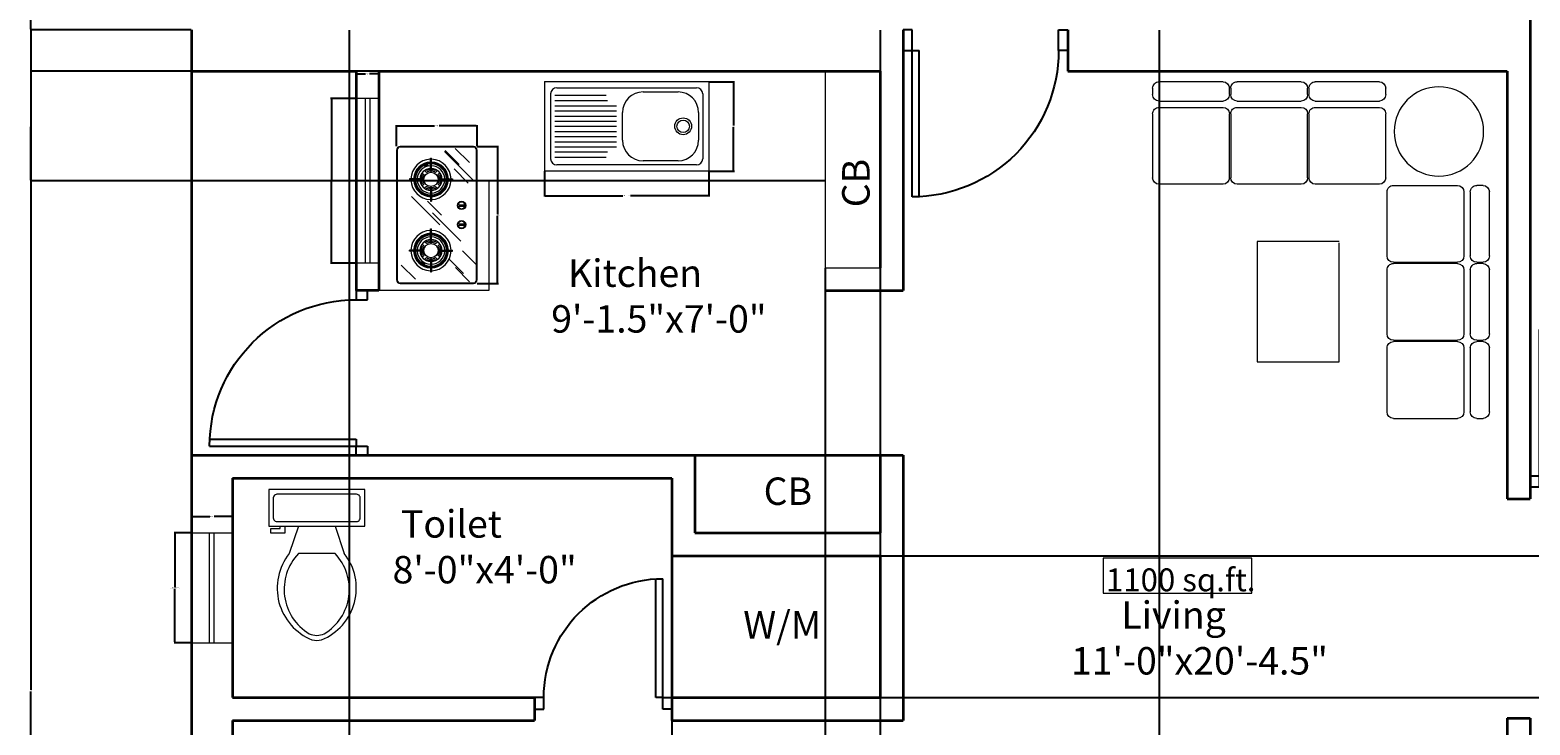
# Model space of a CAD drawing. Units: inches. Extents: x 3198 to 3702, y 1509 to 2253.
# Tile 2 of 6: x 3198 to 3526, y 1693 to 1845. Entities that reach past the tile are written whole.
import ezdxf

# ---------------------------------------------------------------- set-up
doc = ezdxf.new("R2010")
doc.units = ezdxf.units.IN
for name, color, linetype, lineweight in [('A-ANNO-DIMS', 2, 'Continuous', 18), ('A-ANNO-TEXT', 7, 'Continuous', 18), ('A-AREA-IDEN', 7, 'Continuous', 18), ('A-DOOR', 3, 'Continuous', 25), ('A-EQPM', 8, 'Continuous', 18), ('A-FLOR-CASE', 9, 'Continuous', 18), ('A-FLOR-FIXT', 9, 'Continuous', 18), ('A-FURN', 8, 'Continuous', 13), ('A-GLAZ', 4, 'Continuous', 18), ('A-WALL', 7, 'Continuous', 35)]:
    doc.layers.add(name, color=color, linetype=linetype, lineweight=lineweight)
doc.styles.get("Standard").update_dxf_attribs({"font": 'arial.ttf'})
doc.dimstyles.get("Standard").update_dxf_attribs({"dimtxt": 0.18, "dimasz": 0.18, "dimexe": 0.18, "dimexo": 0.0625, "dimgap": 0.09, "dimtad": 0, "dimtih": 1, "dimtoh": 1, "dimdec": 4, "dimzin": 0, "dimdsep": 46, "dimtxsty": 'Standard', "dimcen": 0.09, "dimadec": 0, "dimazin": 0, "dimtfac": 1, "dimtdec": 4, "dimtofl": 0, "dimtmove": 0, "dimatfit": 3, "dimfxl": 1, "dimtolj": 1, "dimtzin": 0, "dimarcsym": 0})

# ---------------------------------------------------------------- blocks, each defined once
blk = doc.blocks.new('A$C753D6792')
at = {"linetype": 'ByBlock'}
for p, q in [((0, 2530), (0, 2580)), ((50, 2630), (550, 2630)), ((600, 2580), (600, 2530)), ((610, 2530), (610, 2580)), ((660, 2630), (1160, 2630)), ((1210, 2580), (1210, 2530)), ((1220, 2530), (1220, 2580)), ((1270, 2630), (1770, 2630)), ((1820, 2580), (1820, 2530)), ((550, 2480), (50, 2480)), ((1160, 2480), (660, 2480)), ((1770, 2480), (1270, 2480)), ((0, 1880), (0, 2380)), ((550, 2430), (50, 2430)), ((600, 2380), (600, 1880)), ((610, 1880), (610, 2380)), ((1160, 2430), (660, 2430)), ((1210, 2380), (1210, 1880)), ((1220, 1880), (1220, 2380)), ((1770, 2430), (1270, 2430)), ((1820, 1880), (1820, 2380)), ((50, 1830), (427, 1830)), ((387, 1830), (550, 1830)), ((660, 1830), (1037, 1830)), ((997, 1830), (1160, 1830)), ((1270, 1830), (1647, 1830)), ((1607, 1830), (1770, 1830)), ((1830, 1770), (1830, 1393)), ((1880, 1820), (2380, 1820)), ((2430, 1270), (2430, 1770)), ((2480, 1270), (2480, 1770)), ((2530, 1820), (2580, 1820)), ((2630, 1770), (2630, 1270)), ((442, 815), (442, 1455)), ((442, 1455), (1372, 1455)), ((1382, 1455), (1382, 815)), ((1830, 1433), (1830, 1270)), ((2380, 1220), (1880, 1220)), ((1880, 1210), (2380, 1210)), ((2580, 1220), (2530, 1220)), ((2530, 1210), (2580, 1210)), ((1830, 1160), (1830, 783)), ((2430, 660), (2430, 1160)), ((2480, 660), (2480, 1160)), ((2630, 1160), (2630, 660)), ((1830, 823), (1830, 660)), ((1382, 815), (442, 815)), ((2380, 610), (1880, 610)), ((1880, 600), (2380, 600)), ((2580, 610), (2530, 610)), ((2530, 600), (2580, 600)), ((1830, 550), (1830, 173)), ((2430, 50), (2430, 550)), ((2480, 50), (2480, 550)), ((2630, 550), (2630, 50)), ((1830, 213), (1830, 50)), ((2380, 0), (1880, 0)), ((2580, 0), (2530, 0))]:
    blk.add_line(p, q, dxfattribs=at)
blk.add_circle((2242, 2235), 349, dxfattribs=at)
for centre, start, end in [((50, 2580), 90, 180), ((550, 2580), 0, 90), ((550, 2580), 0, 90), ((660, 2580), 90, 180), ((1160, 2580), 0, 90), ((1160, 2580), 0, 90), ((1270, 2580), 90, 180), ((1770, 2580), 0, 90), ((1770, 2580), 0, 90), ((50, 2530), 180, 270), ((550, 2530), 270, 0), ((550, 2530), 270, 0), ((660, 2530), 180, 270), ((1160, 2530), 270, 0), ((1160, 2530), 270, 0), ((1270, 2530), 180, 270), ((1770, 2530), 270, 0), ((1770, 2530), 270, 0), ((50, 2380), 90, 180), ((550, 2380), 0, 90), ((550, 2380), 0, 90), ((660, 2380), 90, 180), ((1160, 2380), 0, 90), ((1160, 2380), 0, 90), ((1270, 2380), 90, 180), ((1770, 2380), 0, 90), ((1770, 2380), 0, 90), ((50, 1880), 180, 270), ((550, 1880), 270, 0), ((660, 1880), 180, 270), ((1160, 1880), 270, 0), ((1270, 1880), 180, 270), ((1770, 1880), 270, 0), ((1880, 1770), 90, 180), ((2380, 1770), 0, 90), ((2530, 1770), 90, 180), ((2580, 1770), 0, 90), ((1880, 1270), 180, 270), ((1880, 1160), 90, 180), ((2380, 1270), 270, 0), ((2380, 1270), 270, 0), ((2380, 1160), 0, 90), ((2530, 1270), 180, 270), ((2530, 1270), 180, 270), ((2530, 1160), 90, 180), ((2580, 1270), 270, 0), ((2580, 1270), 270, 0), ((2580, 1160), 0, 90), ((1880, 660), 180, 270), ((1880, 550), 90, 180), ((2380, 660), 270, 0), ((2380, 660), 270, 0), ((2380, 550), 0, 90), ((2530, 660), 180, 270), ((2530, 660), 180, 270), ((2530, 550), 90, 180), ((2580, 660), 270, 0), ((2580, 660), 270, 0), ((2580, 550), 0, 90), ((1880, 50), 180, 270), ((2380, 50), 270, 0), ((2380, 50), 270, 0), ((2530, 50), 180, 270), ((2530, 50), 180, 270), ((2580, 50), 270, 0), ((2580, 50), 270, 0)]:
    blk.add_arc(centre, 50, start, end, dxfattribs=at)
blk = doc.blocks.new('A$C48FA29D1')
for p, q in [((23.9, 336.8), (101.3, 414.2)), ((177.6, 369.5), (182.6, 369.5)), ((320.9, 202.7), (475.7, 357.5)), ((572.4, 369.5), (567.4, 369.5)), ((63.2, 254.2), (63.2, 249.2)), ((299, 254.2), (299, 249.2)), ((374.2, 193.8), (451.6, 271.2)), ((451, 254.2), (451, 249.2)), ((686.8, 254.2), (686.8, 249.2)), ((232.1, 89.3), (386.9, 244.1)), ((567.6, 22.2), (722.4, 177)), ((650.5, 97.2), (727.9, 174.6)), ((10.1, 41), (87.5, 118.4)), ((54.5, 73.5), (131.9, 150.9)), ((177.6, 133.3), (182.6, 133.3)), ((549.9, 47.9), (627.2, 125.3)), ((572.4, 133.3), (567.4, 133.3)), ((661.4, 42), (738.7, 119.3)), ((100.9, 1.5), (178.3, 78.9))]:
    blk.add_line(p, q)
at = {"ltscale": 0.18}
for p, q in [((177.6, 296.7), (177.6, 369.5)), ((182.6, 296.7), (182.6, 369.5)), ((567.4, 296.7), (567.4, 369.5)), ((572.4, 296.7), (572.4, 369.5)), ((135.1, 254.2), (63.2, 254.2)), ((135.1, 249.2), (63.2, 249.2)), ((126.9, 279.5), (132.1, 274.3)), ((131.2, 286.5), (142, 275.7)), ((145.3, 300.6), (156.1, 289.8)), ((152.3, 304.9), (157.6, 299.7)), ((202.6, 299.7), (207.8, 304.9)), ((204, 289.8), (214.8, 300.6)), ((218.2, 275.7), (229, 286.5)), ((225, 254.2), (299, 254.2)), ((225, 249.2), (299, 249.2)), ((228.1, 274.3), (233.3, 279.5)), ((525, 254.2), (451, 254.2)), ((525, 249.2), (451, 249.2)), ((521.9, 274.3), (516.7, 279.5)), ((531.8, 275.7), (521, 286.5)), ((546, 289.8), (535.2, 300.6)), ((547.4, 299.7), (542.2, 304.9)), ((597.7, 304.9), (592.4, 299.7)), ((604.7, 300.6), (593.9, 289.8)), ((618.8, 286.5), (608, 275.7)), ((614.9, 254.2), (686.8, 254.2)), ((614.9, 249.2), (686.8, 249.2)), ((623.1, 279.5), (617.9, 274.3)), ((126.9, 224), (132.1, 229.2)), ((131.2, 217), (142, 227.8)), ((145.3, 202.8), (156.1, 213.6)), ((152.3, 198.5), (157.6, 203.8)), ((177.6, 206.8), (177.6, 133.3)), ((182.6, 206.8), (182.6, 133.3)), ((202.6, 203.8), (207.8, 198.5)), ((204, 213.6), (214.8, 202.8)), ((218.2, 227.8), (229, 217)), ((228.1, 229.2), (233.3, 224)), ((521.9, 229.2), (516.7, 224)), ((531.8, 227.8), (521, 217)), ((546, 213.6), (535.2, 202.8)), ((547.4, 203.8), (542.2, 198.5)), ((567.4, 206.8), (567.4, 133.3)), ((572.4, 206.8), (572.4, 133.3)), ((597.7, 198.5), (592.4, 203.8)), ((604.7, 202.8), (593.9, 213.6)), ((618.8, 217), (608, 227.8)), ((623.1, 224), (617.9, 229.2)), ((318.6, 99.8), (318.6, 69)), ((326.6, 99.8), (326.6, 69)), ((423.4, 99.8), (423.4, 69)), ((431.4, 99.8), (431.4, 69))]:
    blk.add_line(p, q, dxfattribs=at)
for points in [[(20, 0), (730, 0, 0.414214), (750, 20), (750, 420, 0.414214), (730, 440), (20, 440, 0.414214), (0, 420), (0, 20, 0.414214)], [(20, 3), (730, 3, 0.414214), (747, 20), (747, 420, 0.414214), (730, 437), (20, 437, 0.414214), (3, 420), (3, 20, 0.414214)]]:
    blk.add_lwpolyline(points, format="xyb", close=True)
for centre in [(109.4, 291.3), (115.3, 300.3), (642.8, 283.6), (646.9, 273)]:
    blk.add_circle(centre, 3.58)
for centre, radius in [((180.1, 251.7), 39), ((569.9, 251.7), 39), ((322.6, 84.4), 22.5), ((322.6, 84.4), 21.5), ((427.4, 84.4), 22.5), ((427.4, 84.4), 21.5)]:
    blk.add_circle(centre, radius, dxfattribs=at)
for centre, radius, start, end in [((180.1, 251.7), 110, 91.30229, 178.69771), ((180.1, 251.7), 95, 91.59175, 178.40825), ((180.1, 251.7), 90, 91.59175, 178.40825), ((180.1, 251.7), 85, 91.68541, 178.31459), ((180.1, 251.7), 110, 1.30229, 88.69771), ((180.1, 251.7), 90, 1.59175, 88.40825), ((180.1, 251.7), 85, 1.68541, 88.31459), ((180.1, 251.7), 95, 1.59175, 88.40825), ((569.9, 251.7), 110, 91.30229, 178.69771), ((569.9, 251.7), 95, 91.59175, 178.40825), ((569.9, 251.7), 90, 91.59175, 178.40825), ((569.9, 251.7), 85, 91.68541, 178.31459), ((569.9, 251.7), 110, 1.30229, 88.69771), ((569.9, 251.7), 90, 1.59175, 88.40825), ((569.9, 251.7), 85, 1.68541, 88.31459), ((569.9, 251.7), 95, 1.59175, 88.40825), ((180.1, 251.7), 110, 181.30229, 268.69771), ((180.1, 251.7), 95, 181.59175, 268.40825), ((180.1, 251.7), 90, 181.59175, 268.40825), ((180.1, 251.7), 85, 181.68541, 268.31459), ((180.1, 251.7), 75, 91.91021, 178.08979), ((180.1, 251.7), 75, 181.91021, 268.08979), ((180.1, 251.7), 60, 92.38802, 177.61198), ((180.1, 251.7), 60, 182.38802, 267.61198), ((180.1, 251.7), 53, 154.85389, 177.29637), ((180.1, 251.7), 53, 182.70363, 205.14611), ((180.1, 251.7), 45, 147.83959, 176.81526), ((134.3, 251.7), 2.64, 288.75105, 71.24895), ((180.1, 251.7), 45, 183.18474, 212.16041), ((180.1, 251.7), 45, 93.18474, 122.16041), ((180.1, 251.7), 53, 92.70363, 115.14611), ((180.1, 297), 2.52, 186.73537, 353.26463), ((180.1, 251.7), 75, 1.91021, 88.08979), ((180.1, 251.7), 60, 2.38802, 87.61198), ((180.1, 251.7), 53, 64.85389, 87.29637), ((180.1, 251.7), 45, 57.83959, 86.81526), ((180.1, 251.7), 90, 271.59175, 358.40825), ((180.1, 251.7), 85, 271.68541, 358.31459), ((180.1, 251.7), 110, 271.30229, 358.69771), ((180.1, 251.7), 75, 271.91021, 358.08979), ((180.1, 251.7), 60, 272.38802, 357.61198), ((180.1, 251.7), 95, 271.59175, 358.40825), ((180.1, 251.7), 45, 3.18474, 32.16041), ((180.1, 251.7), 45, 327.83959, 356.81526), ((225.9, 251.7), 2.67, 110.55069, 249.44931), ((180.1, 251.7), 53, 2.70363, 25.14611), ((180.1, 251.7), 53, 334.85389, 357.29637), ((569.9, 251.7), 110, 181.30229, 268.69771), ((569.9, 251.7), 95, 181.59175, 268.40825), ((569.9, 251.7), 90, 181.59175, 268.40825), ((569.9, 251.7), 85, 181.68541, 268.31459), ((569.9, 251.7), 75, 91.91021, 178.08979), ((569.9, 251.7), 75, 181.91021, 268.08979), ((569.9, 251.7), 60, 92.38802, 177.61198), ((569.9, 251.7), 60, 182.38802, 267.61198), ((569.9, 251.7), 53, 154.85389, 177.29637), ((569.9, 251.7), 53, 182.70363, 205.14611), ((569.9, 251.7), 45, 147.83959, 176.81526), ((524.2, 251.7), 2.63, 288.41197, 71.58803), ((569.9, 251.7), 45, 183.18474, 212.16041), ((569.9, 251.7), 45, 93.18474, 122.16041), ((569.9, 251.7), 53, 92.70363, 115.14611), ((569.9, 296.8), 2.51, 183.95793, 356.04207), ((569.9, 251.7), 75, 1.91021, 88.08979), ((569.9, 251.7), 60, 2.38802, 87.61198), ((569.9, 251.7), 53, 64.85389, 87.29637), ((569.9, 251.7), 45, 57.83959, 86.81526), ((569.9, 251.7), 75, 271.91021, 358.08979), ((569.9, 251.7), 85, 271.68541, 358.31459), ((569.9, 251.7), 110, 271.30229, 358.69771), ((569.9, 251.7), 90, 271.59175, 358.40825), ((569.9, 251.7), 60, 272.38802, 357.61198), ((569.9, 251.7), 95, 271.59175, 358.40825), ((569.9, 251.7), 45, 3.18474, 32.16041), ((569.9, 251.7), 45, 327.83959, 356.81526), ((615.5, 251.7), 2.58, 104.29448, 255.70552), ((569.9, 251.7), 53, 2.70363, 25.14611), ((569.9, 251.7), 53, 334.85389, 357.29637), ((180.1, 251.7), 45, 237.83959, 266.81526), ((180.1, 251.7), 53, 244.85389, 267.29637), ((180.1, 205.8), 2.69, 21.78852, 158.21148), ((180.1, 251.7), 45, 273.18474, 302.16041), ((180.1, 251.7), 53, 272.70363, 295.14611), ((569.9, 251.7), 45, 237.83959, 266.81526), ((569.9, 251.7), 53, 244.85389, 267.29637), ((569.9, 206), 2.63, 17.9418, 162.0582), ((569.9, 251.7), 45, 273.18474, 302.16041), ((569.9, 251.7), 53, 272.70363, 295.14611), ((322.6, 84.4), 18.5, 111.32369, 248.67631), ((316.6, 99.8), 2, 0, 111.32369), ((328.6, 99.8), 2, 68.67631, 180), ((322.6, 84.4), 18.5, 291.32369, 68.67631), ((427.4, 84.4), 18.5, 111.32369, 248.67631), ((421.4, 99.8), 2, 0, 111.32369), ((433.4, 99.8), 2, 68.67631, 180), ((427.4, 84.4), 18.5, 291.32369, 68.67631), ((316.6, 69), 2, 248.67631, 0), ((328.6, 69), 2, 180, 291.32369), ((421.4, 69), 2, 248.67631, 0), ((433.4, 69), 2, 180, 291.32369)]:
    blk.add_arc(centre, radius, start, end, dxfattribs=at)
blk = doc.blocks.new('A$C56104318')
for p, q in [((0, 0.609), (1.12, 0.609)), ((0, 0.609), (0, 0)), ((0.042, 0.525), (0.042, 0.084)), ((0.42, 0.515), (0.07, 0.515)), ((0.084, 0.567), (1.036, 0.567)), ((0.672, 0.539), (0.91, 0.539)), ((1.078, 0.525), (1.078, 0.084)), ((1.12, 0.609), (1.12, 0)), ((0.07, 0.48), (0.429, 0.48)), ((0.07, 0.445), (0.49, 0.445)), ((0.07, 0.41), (0.49, 0.41)), ((0.07, 0.375), (0.49, 0.375)), ((0.07, 0.34), (0.49, 0.34)), ((0.532, 0.21), (0.532, 0.399)), ((1.05, 0.399), (1.05, 0.21)), ((0.07, 0.305), (0.49, 0.305)), ((0.07, 0.27), (0.49, 0.27)), ((0.07, 0.235), (0.49, 0.235)), ((0.07, 0.2), (0.49, 0.2)), ((0.07, 0.165), (0.49, 0.165)), ((0.07, 0.13), (0.429, 0.13)), ((0.07, 0.094), (0.42, 0.094)), ((1.036, 0.042), (0.084, 0.042)), ((0.91, 0.07), (0.672, 0.07)), ((1.12, 0), (0, 0))]:
    blk.add_line(p, q)
for radius in [0.0574, 0.0427]:
    blk.add_circle((0.945, 0.305), radius)
for centre, radius, start, end in [((0.084, 0.525), 0.042, 90, 180), ((0.672, 0.399), 0.14, 90, 180), ((0.91, 0.399), 0.14, 0, 90), ((1.036, 0.525), 0.042, 0, 90), ((0.672, 0.21), 0.14, 180, 270), ((0.91, 0.21), 0.14, 270, 0), ((0.084, 0.084), 0.042, 180, 270), ((1.036, 0.084), 0.042, 270, 0)]:
    blk.add_arc(centre, radius, start, end)
blk = doc.blocks.new('A$C559B0E78')
at = {"xscale": 729, "yscale": 729, "zscale": 729}
blk.add_blockref('A$C56104318', (0, 0), dxfattribs=at)
blk = doc.blocks.new('*U4')
for p, q in [((9.5, -6), (9.5, -2)), ((-10, -8.5), (-8, -8.5)), ((-10, -9.5), (-10, -8.5)), ((-7, -9.5), (-10, -9.5)), ((-8, -8.5), (-8, -8)), ((-7, -8), (-7, -9.5)), ((-4, -8), (-6, -14)), ((4, -8), (6, -14)), ((4, -14), (-4, -14))]:
    blk.add_line(p, q)
blk.add_lwpolyline([(10.5, -8), (10.5, 0), (-10.5, 0), (-10.5, -8)], close=True)
for points in [[(-9.5, -2), (-9.5, -6)], [(8.5, -1), (-8.5, -1)], [(-8.5, -7), (8.5, -7)]]:
    blk.add_lwpolyline(points)
for centre, radius, start, end in [((-8.62, -1.88), 0.884, 81.8699, 188.1301), ((8.62, -1.88), 0.884, 351.8699, 98.1301), ((-8.62, -6.12), 0.884, 171.8699, 278.1301), ((8.62, -6.12), 0.884, 261.8699, 8.1301), ((3.52, -21.58), 12.17, 141.4691, 247.9714), ((4.2, -21.82), 11.33, 136.3677, 238.9468), ((-3.52, -21.58), 12.17, 292.0284, 38.5307), ((-4.2, -21.82), 11.33, 301.053, 43.6321), ((0, -27.88), 4, 245.7318, 294.2682), ((0, -29), 4, 254.8605, 285.1395)]:
    blk.add_arc(centre, radius, start, end)
blk = doc.blocks.new('DOOR-SINGLE-32')
for p, q in [((0, 34), (32, 34)), ((32, 36), (32, 34)), ((32, 34), (34.5, 34)), ((32, 32.5), (32, 34)), ((34.5, 34), (34.5, 36)), ((0.04, 32.5), (32, 32.5)), ((32, 0), (32, 2)), ((32, 2), (34.5, 2)), ((34.5, 2), (34.5, 0))]:
    blk.add_line(p, q)
blk.add_arc((32, 34), 32, 180, 270)
blk = doc.blocks.new('DOOR-SINGLE-26')
for p, q in [((0, 30), (0, 28)), ((2.5, 28), (2.5, 30)), ((0, 28), (2.5, 28)), ((2.5, 28), (28.5, 28)), ((2.5, 28), (2.5, 26.5)), ((2.5, 26.5), (28.46, 26.5)), ((0, 0), (0, 2)), ((0, 2), (2.5, 2)), ((2.5, 2), (2.5, 0))]:
    blk.add_line(p, q)
blk.add_arc((2.5, 28), 26, 270, 0)
blk = doc.blocks.new('DOOR-ENTRY-32')
for p, q in [((2, 36.5), (2, 4.5)), ((3.5, 36.46), (3.5, 4.5)), ((0, 4.5), (2, 4.5)), ((2, 4.5), (2, 0)), ((2, 4.5), (3.5, 4.5)), ((36, 4.5), (34, 4.5)), ((34, 4.5), (34, 0)), ((2, 0), (0, 0)), ((34, 0), (36, 0))]:
    blk.add_line(p, q)
blk.add_arc((2, 4.5), 32, 360, 90)
blk = doc.blocks.new('WIN-24-W9')
for p, q in [((9, 24), (0, 24)), ((4, 24), (4, 0)), ((5, 24), (5, 0)), ((9, 0), (0, 0))]:
    blk.add_line(p, q)
blk = doc.blocks.new('WIN-36-W5')
for p, q in [((0, 36), (5, 36)), ((2, 0), (2, 36)), ((3, 0), (3, 36)), ((0, 0), (5, 0))]:
    blk.add_line(p, q)
blk = doc.blocks.new('*D25')
at = {"layer": 'A-ANNO-DIMS', "color": 0, "lineweight": -2, "transparency": 16777216}
for p, q in [((3232.98, 1734.89), (3229.27, 1734.89)), ((3229.45, 1734.71), (3229.45, 1723.07)), ((3229.45, 1711.07), (3229.45, 1722.7)), ((3232.98, 1710.89), (3229.27, 1710.89))]:
    blk.add_line(p, q, dxfattribs=at)
at = {"layer": 'A-ANNO-DIMS', "color": 0, "transparency": 16777216}
for points in [[(3229.42, 1734.71), (3229.48, 1734.71), (3229.45, 1734.89)], [(3229.42, 1711.07), (3229.48, 1711.07), (3229.45, 1710.89)]]:
    blk.add_solid(points, dxfattribs=at)
at = {"layer": 'Defpoints', "color": 0, "transparency": 16777216}
for p in [(3233.05, 1734.89), (3229.45, 1710.89), (3233.05, 1710.89)]:
    blk.add_point(p, dxfattribs=at)
at = {"layer": 'A-ANNO-DIMS', "color": 0, "transparency": 16777216, "insert": (3229.45, 1722.89), "char_height": 0.18, "attachment_point": 5}
blk.add_mtext('\\A1;WINDOW 24 TYP.', dxfattribs=at)
blk = doc.blocks.new('*D26')
at = {"layer": 'A-ANNO-DIMS', "color": 0, "lineweight": -2, "transparency": 16777216}
for p, q in [((3233.05, 1734.95), (3233.05, 1738.67)), ((3233.23, 1738.49), (3237.09, 1738.49)), ((3241.87, 1738.49), (3238.01, 1738.49)), ((3242.05, 1734.95), (3242.05, 1738.67))]:
    blk.add_line(p, q, dxfattribs=at)
at = {"layer": 'A-ANNO-DIMS', "color": 0, "transparency": 16777216}
for points in [[(3233.23, 1738.52), (3233.23, 1738.46), (3233.05, 1738.49)], [(3241.87, 1738.52), (3241.87, 1738.46), (3242.05, 1738.49)]]:
    blk.add_solid(points, dxfattribs=at)
at = {"layer": 'Defpoints', "color": 0, "transparency": 16777216}
for p in [(3233.05, 1738.49), (3233.05, 1734.89), (3242.05, 1734.89)]:
    blk.add_point(p, dxfattribs=at)
at = {"layer": 'A-ANNO-DIMS', "color": 0, "transparency": 16777216, "insert": (3237.55, 1738.49), "char_height": 0.18, "attachment_point": 5}
blk.add_mtext('\\A1;9 TYP.', dxfattribs=at)
blk = doc.blocks.new('*D33')
at = {"layer": 'A-ANNO-DIMS', "color": 0, "lineweight": -2, "transparency": 16777216}
for p, q in [((3295.53, 1819.41), (3300.15, 1819.41)), ((3299.97, 1819.23), (3299.97, 1804.61)), ((3299.97, 1789.62), (3299.97, 1804.24)), ((3295.53, 1789.44), (3300.15, 1789.44))]:
    blk.add_line(p, q, dxfattribs=at)
at = {"layer": 'A-ANNO-DIMS', "color": 0, "transparency": 16777216}
for points in [[(3299.94, 1819.23), (3300, 1819.23), (3299.97, 1819.41)], [(3299.94, 1789.62), (3300, 1789.62), (3299.97, 1789.44)]]:
    blk.add_solid(points, dxfattribs=at)
at = {"layer": 'Defpoints', "color": 0, "transparency": 16777216}
for p in [(3295.47, 1819.41), (3299.97, 1819.41), (3295.47, 1789.44)]:
    blk.add_point(p, dxfattribs=at)
at = {"layer": 'A-ANNO-DIMS', "color": 0, "transparency": 16777216, "insert": (3299.97, 1804.42), "char_height": 0.18, "attachment_point": 5}
blk.add_mtext('\\A1;HOB 30 TYP.', dxfattribs=at)
blk = doc.blocks.new('*D34')
at = {"layer": 'A-ANNO-DIMS', "color": 0, "lineweight": -2, "transparency": 16777216}
for p, q in [((3277.88, 1819.47), (3277.88, 1824.09)), ((3278.06, 1823.91), (3286.16, 1823.91)), ((3295.29, 1823.91), (3287.2, 1823.91)), ((3295.47, 1819.47), (3295.47, 1824.09))]:
    blk.add_line(p, q, dxfattribs=at)
at = {"layer": 'A-ANNO-DIMS', "color": 0, "transparency": 16777216}
for points in [[(3278.06, 1823.94), (3278.06, 1823.88), (3277.88, 1823.91)], [(3295.29, 1823.94), (3295.29, 1823.88), (3295.47, 1823.91)]]:
    blk.add_solid(points, dxfattribs=at)
at = {"layer": 'Defpoints', "color": 0, "transparency": 16777216}
for p in [(3277.88, 1823.91), (3277.88, 1819.41), (3295.47, 1819.41)]:
    blk.add_point(p, dxfattribs=at)
at = {"layer": 'A-ANNO-DIMS', "color": 0, "transparency": 16777216, "insert": (3286.68, 1823.91), "char_height": 0.18, "attachment_point": 5}
blk.add_mtext('\\A1;18 TYP.', dxfattribs=at)
blk = doc.blocks.new('*D35')
at = {"layer": 'A-ANNO-DIMS', "color": 0, "lineweight": -2, "transparency": 16777216}
for p, q in [((3310.19, 1813.98), (3310.19, 1808.47)), ((3346.13, 1813.98), (3346.13, 1808.47)), ((3310.37, 1808.65), (3327.31, 1808.65)), ((3345.95, 1808.65), (3329.02, 1808.65))]:
    blk.add_line(p, q, dxfattribs=at)
at = {"layer": 'A-ANNO-DIMS', "color": 0, "transparency": 16777216}
for points in [[(3310.37, 1808.68), (3310.37, 1808.62), (3310.19, 1808.65)], [(3345.95, 1808.68), (3345.95, 1808.62), (3346.13, 1808.65)]]:
    blk.add_solid(points, dxfattribs=at)
at = {"layer": 'Defpoints', "color": 0, "transparency": 16777216}
for p in [(3310.19, 1814.04), (3346.13, 1814.04), (3346.13, 1808.65)]:
    blk.add_point(p, dxfattribs=at)
at = {"layer": 'A-ANNO-DIMS', "color": 0, "transparency": 16777216, "insert": (3328.16, 1808.65), "char_height": 0.18, "attachment_point": 5}
blk.add_mtext('\\A1;SINK 36 TYP.', dxfattribs=at)
blk = doc.blocks.new('*D36')
at = {"layer": 'A-ANNO-DIMS', "color": 0, "lineweight": -2, "transparency": 16777216}
for p, q in [((3346.2, 1833.58), (3351.7, 1833.58)), ((3351.52, 1833.4), (3351.52, 1823.99)), ((3351.52, 1814.22), (3351.52, 1823.63)), ((3346.2, 1814.04), (3351.7, 1814.04))]:
    blk.add_line(p, q, dxfattribs=at)
at = {"layer": 'A-ANNO-DIMS', "color": 0, "transparency": 16777216}
for points in [[(3351.49, 1833.4), (3351.55, 1833.4), (3351.52, 1833.58)], [(3351.49, 1814.22), (3351.55, 1814.22), (3351.52, 1814.04)]]:
    blk.add_solid(points, dxfattribs=at)
at = {"layer": 'Defpoints', "color": 0, "transparency": 16777216}
for p in [(3346.13, 1833.58), (3351.52, 1833.58), (3346.13, 1814.04)]:
    blk.add_point(p, dxfattribs=at)
at = {"layer": 'A-ANNO-DIMS', "color": 0, "transparency": 16777216, "insert": (3351.52, 1823.81), "char_height": 0.18, "attachment_point": 5}
blk.add_mtext('\\A1;20 TYP.', dxfattribs=at)
blk = doc.blocks.new('*D41')
at = {"layer": 'A-ANNO-DIMS', "color": 0, "lineweight": -2, "transparency": 16777216}
for p, q in [((3268.98, 1829.89), (3263.47, 1829.89)), ((3263.65, 1829.71), (3263.65, 1812.07)), ((3263.65, 1794.07), (3263.65, 1811.7)), ((3268.98, 1793.89), (3263.47, 1793.89))]:
    blk.add_line(p, q, dxfattribs=at)
at = {"layer": 'A-ANNO-DIMS', "color": 0, "transparency": 16777216}
for points in [[(3263.62, 1829.71), (3263.68, 1829.71), (3263.65, 1829.89)], [(3263.62, 1794.07), (3263.68, 1794.07), (3263.65, 1793.89)]]:
    blk.add_solid(points, dxfattribs=at)
at = {"layer": 'Defpoints', "color": 0, "transparency": 16777216}
for p in [(3269.05, 1829.89), (3263.65, 1793.89), (3269.05, 1793.89)]:
    blk.add_point(p, dxfattribs=at)
at = {"layer": 'A-ANNO-DIMS', "color": 0, "transparency": 16777216, "insert": (3263.65, 1811.89), "char_height": 0.18, "attachment_point": 5}
blk.add_mtext('\\A1;KITCHEN WINDOW 36 TYP.', dxfattribs=at)
blk = doc.blocks.new('*D42')
at = {"layer": 'A-ANNO-DIMS', "color": 0, "lineweight": -2, "transparency": 16777216}
for p, q in [((3269.05, 1829.95), (3269.05, 1835.47)), ((3274.05, 1829.95), (3274.05, 1835.47)), ((3269.23, 1835.29), (3271.09, 1835.29)), ((3273.87, 1835.29), (3272.01, 1835.29))]:
    blk.add_line(p, q, dxfattribs=at)
at = {"layer": 'A-ANNO-DIMS', "color": 0, "transparency": 16777216}
for points in [[(3269.23, 1835.32), (3269.23, 1835.26), (3269.05, 1835.29)], [(3273.87, 1835.32), (3273.87, 1835.26), (3274.05, 1835.29)]]:
    blk.add_solid(points, dxfattribs=at)
at = {"layer": 'Defpoints', "color": 0, "transparency": 16777216}
for p in [(3269.05, 1835.29), (3269.05, 1829.89), (3274.05, 1829.89)]:
    blk.add_point(p, dxfattribs=at)
at = {"layer": 'A-ANNO-DIMS', "color": 0, "transparency": 16777216, "insert": (3271.55, 1835.29), "char_height": 0.18, "attachment_point": 5}
blk.add_mtext('\\A1;5 TYP.', dxfattribs=at)
blk = doc.blocks.new('*D49')
at = {"layer": 'A-ANNO-DIMS', "color": 0, "lineweight": -2, "transparency": 16777216}
for p, q in [((3232.98, 1916.89), (3197.82, 1916.89)), ((3198, 1916.71), (3198, 1881.07)), ((3198, 1845.07), (3198, 1880.71)), ((3232.98, 1844.89), (3197.82, 1844.89))]:
    blk.add_line(p, q, dxfattribs=at)
at = {"layer": 'A-ANNO-DIMS', "color": 0, "transparency": 16777216}
for points in [[(3197.97, 1916.71), (3198.03, 1916.71), (3198, 1916.89)], [(3197.97, 1845.07), (3198.03, 1845.07), (3198, 1844.89)]]:
    blk.add_solid(points, dxfattribs=at)
at = {"layer": 'Defpoints', "color": 0, "transparency": 16777216}
for p in [(3233.05, 1916.89), (3198, 1844.89), (3233.05, 1844.89)]:
    blk.add_point(p, dxfattribs=at)
at = {"layer": 'A-ANNO-DIMS', "color": 0, "transparency": 16777216, "insert": (3198, 1880.89), "char_height": 0.18, "attachment_point": 5}
blk.add_mtext('\\A1;72', dxfattribs=at)
blk = doc.blocks.new('*D50')
at = {"layer": 'A-ANNO-DIMS', "color": 0, "lineweight": -2, "transparency": 16777216}
for p, q in [((3232.98, 1844.89), (3197.82, 1844.89)), ((3198, 1844.71), (3198, 1700.57)), ((3198, 1556.07), (3198, 1700.21)), ((3232.98, 1555.89), (3197.82, 1555.89))]:
    blk.add_line(p, q, dxfattribs=at)
at = {"layer": 'A-ANNO-DIMS', "color": 0, "transparency": 16777216}
for points in [[(3197.97, 1844.71), (3198.03, 1844.71), (3198, 1844.89)], [(3197.97, 1556.07), (3198.03, 1556.07), (3198, 1555.89)]]:
    blk.add_solid(points, dxfattribs=at)
at = {"layer": 'Defpoints', "color": 0, "transparency": 16777216}
for p in [(3233.05, 1844.89), (3198, 1555.89), (3233.05, 1555.89)]:
    blk.add_point(p, dxfattribs=at)
at = {"layer": 'A-ANNO-DIMS', "color": 0, "transparency": 16777216, "insert": (3198, 1700.39), "char_height": 0.18, "attachment_point": 5}
blk.add_mtext('\\A1;289', dxfattribs=at)
blk = doc.blocks.new('*D51')
at = {"layer": 'A-ANNO-DIMS', "color": 0, "lineweight": -2, "transparency": 16777216}
for p, q in [((3267.55, 1844.83), (3267.55, 1509.16)), ((3383.55, 1844.83), (3383.55, 1509.16)), ((3267.73, 1509.34), (3325.27, 1509.34)), ((3383.37, 1509.34), (3325.83, 1509.34))]:
    blk.add_line(p, q, dxfattribs=at)
at = {"layer": 'A-ANNO-DIMS', "color": 0, "transparency": 16777216}
for points in [[(3267.73, 1509.37), (3267.73, 1509.31), (3267.55, 1509.34)], [(3383.37, 1509.37), (3383.37, 1509.31), (3383.55, 1509.34)]]:
    blk.add_solid(points, dxfattribs=at)
at = {"layer": 'Defpoints', "color": 0, "transparency": 16777216}
for p in [(3267.55, 1844.89), (3383.55, 1844.89), (3383.55, 1509.34)]:
    blk.add_point(p, dxfattribs=at)
at = {"layer": 'A-ANNO-DIMS', "color": 0, "transparency": 16777216, "insert": (3325.55, 1509.34), "char_height": 0.18, "attachment_point": 5}
blk.add_mtext('\\A1;116', dxfattribs=at)
blk = doc.blocks.new('*D52')
at = {"layer": 'A-ANNO-DIMS', "color": 0, "lineweight": -2, "transparency": 16777216}
for p, q in [((3383.55, 1844.83), (3383.55, 1509.16)), ((3444.55, 1844.83), (3444.55, 1509.16)), ((3383.73, 1509.34), (3413.85, 1509.34)), ((3444.37, 1509.34), (3414.25, 1509.34))]:
    blk.add_line(p, q, dxfattribs=at)
at = {"layer": 'A-ANNO-DIMS', "color": 0, "transparency": 16777216}
for points in [[(3383.73, 1509.37), (3383.73, 1509.31), (3383.55, 1509.34)], [(3444.37, 1509.37), (3444.37, 1509.31), (3444.55, 1509.34)]]:
    blk.add_solid(points, dxfattribs=at)
at = {"layer": 'Defpoints', "color": 0, "transparency": 16777216}
for p in [(3383.55, 1844.89), (3444.55, 1844.89), (3444.55, 1509.34)]:
    blk.add_point(p, dxfattribs=at)
at = {"layer": 'A-ANNO-DIMS', "color": 0, "transparency": 16777216, "insert": (3414.05, 1509.34), "char_height": 0.18, "attachment_point": 5}
blk.add_mtext('\\A1;61', dxfattribs=at)
blk = doc.blocks.new('*D57')
at = {"layer": 'A-ANNO-DIMS', "color": 0, "lineweight": -2, "transparency": 16777216}
for p, q in [((3338.05, 1698.83), (3338.05, 1509.16)), ((3383.55, 1698.83), (3383.55, 1509.16)), ((3338.23, 1509.34), (3360.47, 1509.34)), ((3383.37, 1509.34), (3361.13, 1509.34))]:
    blk.add_line(p, q, dxfattribs=at)
at = {"layer": 'A-ANNO-DIMS', "color": 0, "transparency": 16777216}
for points in [[(3338.23, 1509.37), (3338.23, 1509.31), (3338.05, 1509.34)], [(3383.37, 1509.37), (3383.37, 1509.31), (3383.55, 1509.34)]]:
    blk.add_solid(points, dxfattribs=at)
at = {"layer": 'Defpoints', "color": 0, "transparency": 16777216}
for p in [(3338.05, 1698.89), (3383.55, 1698.89), (3383.55, 1509.34)]:
    blk.add_point(p, dxfattribs=at)
at = {"layer": 'A-ANNO-DIMS', "color": 0, "transparency": 16777216, "insert": (3360.8, 1509.34), "char_height": 0.18, "attachment_point": 5}
blk.add_mtext('\\A1;45.5', dxfattribs=at)
blk = doc.blocks.new('*D58')
at = {"layer": 'A-ANNO-DIMS', "color": 0, "lineweight": -2, "transparency": 16777216}
for p, q in [((3383.61, 1729.89), (3701.78, 1729.89)), ((3701.6, 1729.71), (3701.6, 1714.57)), ((3701.6, 1699.07), (3701.6, 1714.21)), ((3383.61, 1698.89), (3701.78, 1698.89))]:
    blk.add_line(p, q, dxfattribs=at)
at = {"layer": 'A-ANNO-DIMS', "color": 0, "transparency": 16777216}
for points in [[(3701.57, 1729.71), (3701.63, 1729.71), (3701.6, 1729.89)], [(3701.57, 1699.07), (3701.63, 1699.07), (3701.6, 1698.89)]]:
    blk.add_solid(points, dxfattribs=at)
at = {"layer": 'Defpoints', "color": 0, "transparency": 16777216}
for p in [(3383.55, 1729.89), (3701.6, 1729.89), (3383.55, 1698.89)]:
    blk.add_point(p, dxfattribs=at)
at = {"layer": 'A-ANNO-DIMS', "color": 0, "transparency": 16777216, "insert": (3701.6, 1714.39), "char_height": 0.18, "attachment_point": 5}
blk.add_mtext('\\A1;31', dxfattribs=at)
blk = doc.blocks.new('*D59')
at = {"layer": 'A-ANNO-DIMS', "color": 0, "lineweight": -2, "transparency": 16777216}
for p, q in [((3371.48, 1835.89), (3197.82, 1835.89)), ((3198, 1835.71), (3198, 1824.07)), ((3198, 1812.07), (3198, 1823.71)), ((3371.48, 1811.89), (3197.82, 1811.89))]:
    blk.add_line(p, q, dxfattribs=at)
at = {"layer": 'A-ANNO-DIMS', "color": 0, "transparency": 16777216}
for points in [[(3197.97, 1835.71), (3198.03, 1835.71), (3198, 1835.89)], [(3197.97, 1812.07), (3198.03, 1812.07), (3198, 1811.89)]]:
    blk.add_solid(points, dxfattribs=at)
at = {"layer": 'Defpoints', "color": 0, "transparency": 16777216}
for p in [(3198, 1835.89), (3371.55, 1835.89), (3371.55, 1811.89)]:
    blk.add_point(p, dxfattribs=at)
at = {"layer": 'A-ANNO-DIMS', "color": 0, "transparency": 16777216, "insert": (3198, 1823.89), "char_height": 0.18, "attachment_point": 5}
blk.add_mtext('\\A1;24', dxfattribs=at)
blk = doc.blocks.new('*D60')
at = {"layer": 'A-ANNO-DIMS', "color": 0, "lineweight": -2, "transparency": 16777216}
for p, q in [((3371.55, 1792.83), (3371.55, 1509.16)), ((3383.55, 1792.83), (3383.55, 1509.16)), ((3371.73, 1509.34), (3377.34, 1509.34)), ((3383.37, 1509.34), (3377.76, 1509.34))]:
    blk.add_line(p, q, dxfattribs=at)
at = {"layer": 'A-ANNO-DIMS', "color": 0, "transparency": 16777216}
for points in [[(3371.73, 1509.37), (3371.73, 1509.31), (3371.55, 1509.34)], [(3383.37, 1509.37), (3383.37, 1509.31), (3383.55, 1509.34)]]:
    blk.add_solid(points, dxfattribs=at)
at = {"layer": 'Defpoints', "color": 0, "transparency": 16777216}
for p in [(3371.55, 1792.89), (3383.55, 1792.89), (3383.55, 1509.34)]:
    blk.add_point(p, dxfattribs=at)
at = {"layer": 'A-ANNO-DIMS', "color": 0, "transparency": 16777216, "insert": (3377.55, 1509.34), "char_height": 0.18, "attachment_point": 5}
blk.add_mtext('\\A1;12', dxfattribs=at)

msp = doc.modelspace()

# ---------------------------------------------------------------- linework, layer by layer
at = {"layer": 'A-AREA-IDEN'}
msp.add_lwpolyline([(3432.2919, 1721.702), (3464.7788, 1721.702), (3464.7788, 1729.4099), (3432.2919, 1729.4099)], close=True, dxfattribs=at)
at = {"layer": 'A-FLOR-CASE'}
for p, q in [((3371.5475, 1835.888), (3371.5475, 1787.888)), ((3298.0475, 1811.888), (3371.5475, 1811.888)), ((3298.0475, 1811.888), (3298.0475, 1787.888)), ((3371.5475, 1792.888), (3383.5475, 1792.888)), ((3298.0475, 1787.888), (3274.0475, 1787.888))]:
    msp.add_line(p, q, dxfattribs=at)
at = {"layer": 'A-WALL'}
for p, q in [((3525.5475, 1876.388), (3525.5475, 1742.388)), ((3233.0475, 1844.888), (3233.0475, 1555.888)), ((3388.5475, 1844.888), (3388.5475, 1787.888)), ((3424.5475, 1844.888), (3424.5475, 1835.888)), ((3233.0475, 1835.888), (3269.0475, 1835.888)), ((3269.0475, 1835.888), (3269.0475, 1787.888)), ((3274.0475, 1835.888), (3274.0475, 1787.888)), ((3274.0475, 1835.888), (3383.5475, 1835.888)), ((3383.5475, 1835.888), (3383.5475, 1792.888)), ((3424.5475, 1835.888), (3520.5475, 1835.888)), ((3520.5475, 1835.888), (3520.5475, 1742.388)), ((3274.0475, 1787.888), (3269.0475, 1787.888)), ((3371.5475, 1787.888), (3388.5475, 1787.888)), ((3233.0475, 1751.888), (3388.5475, 1751.888)), ((3343.0475, 1751.888), (3343.0475, 1734.888)), ((3383.5475, 1751.888), (3383.5475, 1734.888)), ((3388.5475, 1751.888), (3388.5475, 1693.888)), ((3242.0475, 1746.888), (3338.0475, 1746.888)), ((3242.0475, 1746.888), (3242.0475, 1698.888)), ((3338.0475, 1746.888), (3338.0475, 1693.888)), ((3520.5475, 1742.388), (3525.5475, 1742.388)), ((3343.0475, 1734.888), (3383.5475, 1734.888)), ((3338.0475, 1729.888), (3383.5475, 1729.888)), ((3383.5475, 1729.888), (3383.5475, 1698.888)), ((3242.0475, 1698.888), (3308.0475, 1698.888)), ((3308.0475, 1698.888), (3308.0475, 1693.888)), ((3338.0475, 1698.888), (3383.5475, 1698.888)), ((3242.0475, 1693.888), (3308.0475, 1693.888)), ((3242.0475, 1693.888), (3242.0475, 1564.888)), ((3338.0475, 1693.888), (3388.5475, 1693.888)), ((3520.5475, 1694.388), (3525.5475, 1694.388)), ((3520.5475, 1694.388), (3520.5475, 1591.388)), ((3525.5475, 1694.388), (3525.5475, 1564.888))]:
    msp.add_line(p, q, dxfattribs=at)

# ---------------------------------------------------------------- block references
at = {"layer": 'A-DOOR', "extrusion": (0, 0, -1), "zscale": -1}
for name, p, rotation in [('DOOR-ENTRY-32', (-3388.547, 1844.888), 180), ('DOOR-SINGLE-32', (-3237.047, 1787.888), 180), ('DOOR-SINGLE-32', (-3561.5475, 1779.3885), 269.9999999999991), ('DOOR-SINGLE-26', (-3308.0475, 1696.3875), 89.99999999999548)]:
    msp.add_blockref(name, p, dxfattribs=dict(at, rotation=rotation))
at = {"layer": 'A-EQPM', "xscale": 0.0399671811988082, "yscale": 0.0399671811988082, "zscale": 0.0399671811988082, "rotation": 90}
msp.add_blockref('A$C48FA29D1', (3295.4705, 1789.4366), dxfattribs=at)
at = {"layer": 'A-FLOR-FIXT', "xscale": 0.0440205214597798, "yscale": 0.0440205214597798, "zscale": 0.0440205214597798}
msp.add_blockref('A$C559B0E78', (3310.1909, 1814.0409), dxfattribs=at)
at = {"layer": 'A-FLOR-FIXT'}
msp.add_blockref('*U4', (3260.4496, 1744.3767), dxfattribs=at)
at = {"layer": 'A-FURN', "xscale": -0.0279847415898772, "yscale": 0.0279847415898772, "zscale": 0.0279847415898772, "rotation": 270}
msp.add_blockref('A$C753D6792', (3443.0969, 1759.9487), dxfattribs=at)
at = {"layer": 'A-GLAZ', "rotation": 180}
for name, p in [('WIN-36-W5', (3274.0479, 1829.888)), ('WIN-24-W9', (3242.0479, 1734.888))]:
    msp.add_blockref(name, p, dxfattribs=at)

# ---------------------------------------------------------------- texts
at = {"layer": 'A-ANNO-TEXT', "insert": (3375.2499, 1806.1123), "char_height": 6, "attachment_point": 1, "rotation": 90}
msp.add_mtext_dynamic_manual_height_columns('CB', width=32.112851, gutter_width=12.5, heights=[0], dxfattribs=at)
at = {"layer": 'A-ANNO-TEXT', "char_height": 6, "attachment_point": 1}
for s, insert in [('CB', (3358.0943, 1747.0238)), ('W/M', (3353.6464, 1717.7923))]:
    msp.add_mtext_dynamic_manual_height_columns(s, width=32.112851, gutter_width=12.5, heights=[0], dxfattribs=dict(at, insert=insert))
at = {"layer": 'A-AREA-IDEN'}
for s, width, insert, char_height, attachment_point in [('  Kitchen\\P9\'-1.5"x7\'-0"', 37.305441, (3311.6808, 1794.7078), 6, 1), (' Toilet\\P8\'-0"x4\'-0"', 32.112851, (3277.0133, 1739.8649), 6, 1), ('1100 sq.ft.', 36.112833, (3432.894, 1722.1396), 5, 7), ('{\\H2.4x;      Living\\P11\'-0"x20\'-4.5"}', 72.249028, (3425.2579, 1703.9324), 2.5, 7)]:
    msp.add_mtext_dynamic_manual_height_columns(s, width=width, gutter_width=12.5, heights=[0], dxfattribs=dict(at, insert=insert, char_height=char_height, attachment_point=attachment_point))

# ---------------------------------------------------------------- dimensions: what is measured, and where the dimension line sits
at = {"layer": 'A-ANNO-DIMS'}
for base, p1, p2, picture, middle in [((3197.9975, 1844.888), (3233.0475, 1916.888), (3233.0475, 1844.888), '*D49', (3197.9975, 1880.888)), ((3197.9975, 1555.888), (3233.0475, 1844.888), (3233.0475, 1555.888), '*D50', (3197.9975, 1700.388)), ((3197.9975, 1835.888), (3371.5475, 1811.888), (3371.5475, 1835.888), '*D59', (3197.9975, 1823.888)), ((3701.5975, 1729.888), (3383.5475, 1698.888), (3383.5475, 1729.888), '*D58', (3701.5975, 1714.388))]:
    dim = msp.add_linear_dim(base=base, p1=p1, p2=p2, angle=90, dimstyle='Standard', override={"dimdec": 0, "dimlfac": 1, "dimrnd": 0, "dimzin": 0, "dimdsep": 46, "dimlunit": 2}, dxfattribs=at)
    dim.commit()
    dim.dimension.update_dxf_attribs({"geometry": picture, "text_midpoint": middle})
for base, p1, p2, override, picture, middle in [((3383.5475, 1509.338), (3267.5475, 1844.888), (3383.5475, 1844.888), {"dimdec": 0, "dimlfac": 1, "dimrnd": 0, "dimzin": 0, "dimdsep": 46, "dimlunit": 2}, '*D51', (3325.5475, 1509.338)), ((3444.5475, 1509.338), (3383.5475, 1844.888), (3444.5475, 1844.888), {"dimdec": 0, "dimlfac": 1, "dimrnd": 0, "dimzin": 0, "dimdsep": 46, "dimlunit": 2}, '*D52', (3414.0475, 1509.338)), ((3383.5475, 1509.338), (3371.5475, 1792.888), (3383.5475, 1792.888), {"dimdec": 0, "dimlfac": 1, "dimrnd": 0, "dimzin": 0, "dimdsep": 46, "dimlunit": 2}, '*D60', (3377.5475, 1509.338)), ((3383.5475, 1509.338), (3338.0475, 1698.888), (3383.5475, 1698.888), {"dimdec": 1, "dimlfac": 1, "dimrnd": 0, "dimzin": 0, "dimdsep": 46, "dimlunit": 2}, '*D57', (3360.7975, 1509.338))]:
    dim = msp.add_linear_dim(base=base, p1=p1, p2=p2, dimstyle='Standard', override=override, dxfattribs=at)
    dim.commit()
    dim.dimension.update_dxf_attribs({"geometry": picture, "text_midpoint": middle})
for base, p1, p2, angle, text, picture, middle in [((3269.0475, 1835.288), (3274.0475, 1829.888), (3269.0475, 1829.888), 180, '<> TYP.', '*D42', (3271.5475, 1835.288)), ((3351.5241, 1833.5843), (3346.1328, 1814.0409), (3346.1328, 1833.5843), 90, '<> TYP.', '*D36', (3351.5241, 1823.8126)), ((3263.6475, 1793.888), (3269.0475, 1829.888), (3269.0475, 1793.888), 270, 'KITCHEN WINDOW <> TYP.', '*D41', (3263.6475, 1811.888)), ((3277.8849, 1823.9083), (3295.4705, 1819.412), (3277.8849, 1819.412), 180, '<> TYP.', '*D34', (3286.6777, 1823.9083)), ((3299.9668, 1819.412), (3295.4705, 1789.4366), (3295.4705, 1819.412), 90, 'HOB <> TYP.', '*D33', (3299.9668, 1804.4243)), ((3233.0475, 1738.488), (3242.0475, 1734.888), (3233.0475, 1734.888), 180, '<> TYP.', '*D26', (3237.5475, 1738.488)), ((3229.4475, 1710.888), (3233.0475, 1734.888), (3233.0475, 1710.888), 270, 'WINDOW <> TYP.', '*D25', (3229.4475, 1722.888))]:
    dim = msp.add_linear_dim(base=base, p1=p1, p2=p2, angle=angle, text=text, dimstyle='Standard', override={"dimdec": 0, "dimlfac": 1, "dimrnd": 0, "dimzin": 0, "dimdsep": 46, "dimlunit": 2}, dxfattribs=at)
    dim.commit()
    dim.dimension.update_dxf_attribs({"geometry": picture, "text_midpoint": middle})
dim = msp.add_linear_dim(base=(3346.1328, 1808.6496), p1=(3310.1909, 1814.0409), p2=(3346.1328, 1814.0409), text='SINK <> TYP.', dimstyle='Standard', override={"dimdec": 0, "dimlfac": 1, "dimrnd": 0, "dimzin": 0, "dimdsep": 46, "dimlunit": 2}, dxfattribs=at)
dim.commit()
dim.dimension.update_dxf_attribs({"geometry": '*D35', "text_midpoint": (3328.1619, 1808.6496)})

doc.saveas('drawing.dxf')
